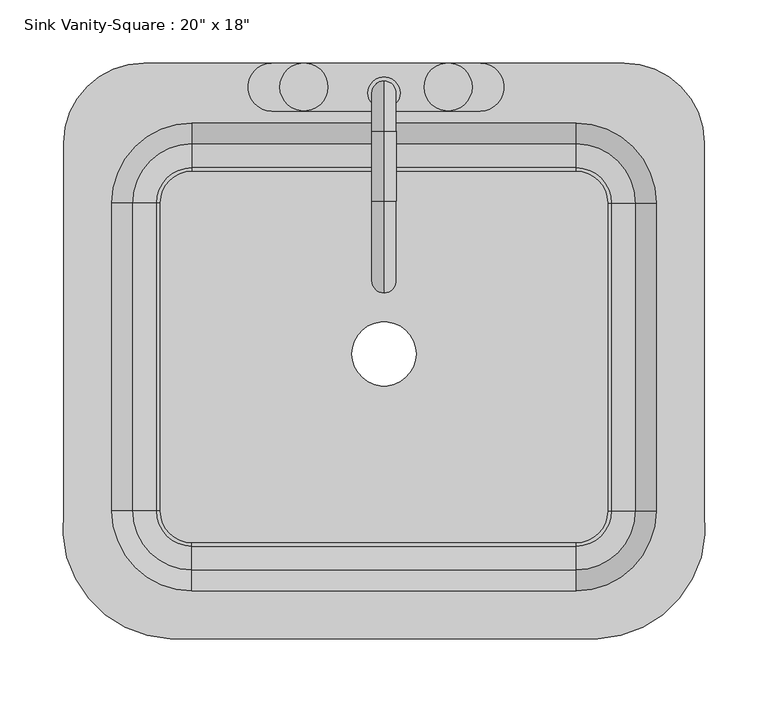
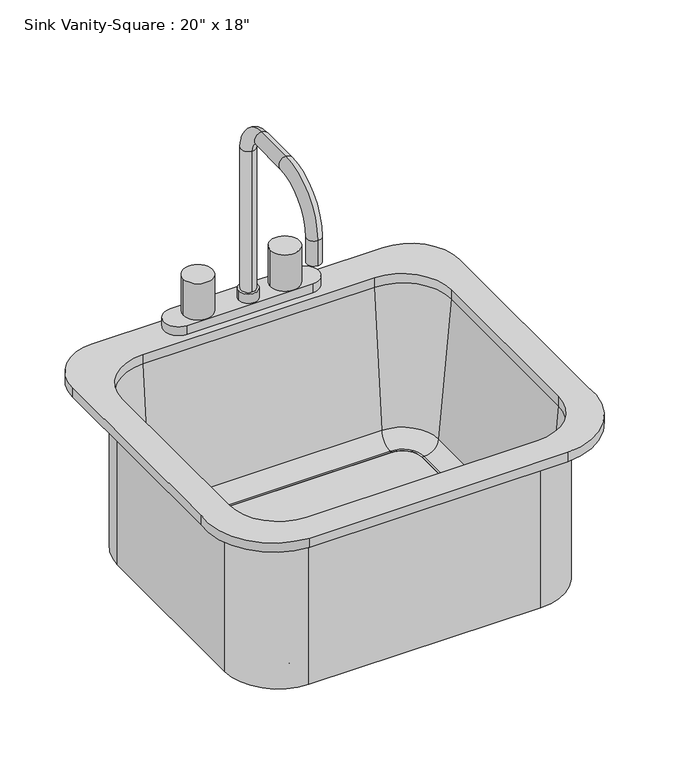
"""IFC4 building model written with IfcOpenShell, lengths in millimetres: flow terminal geometry."""

from ifc_helpers import new_model, si_unit, point, frame, frame_2d, origin, place, context, project, spatial, polyline, circle_curve, ellipse_curve, trimmed, segment, composite_curve, outline, extrude, source, transform, mapped, element, save
from ifc_brep_helpers import plane_surface, cylinder_surface, revolved_surface, advanced_brep


def flow_terminal_62a433f7(model_context):
    return source(origin(), model_context, "Body", "SolidModel", [
        advanced_brep(
        [(-153.9606923, -277.0545989, 800.1), (185.3391735, -277.0545989, 800.1), (269.6892406, -175.4545989, 800.1), (269.6892406, 116.6454011, 800.1), (206.1892406, 180.1454011, 800.1), (-174.8107593, 180.1454011, 800.1), (-238.3107593, 116.6454011, 800.1), (-238.3107593, -175.4545982, 800.1), (168.0892406, 132.5204011, 800.1), (231.5892406, 69.0204011, 800.1), (231.5892406, -175.4545989, 800.1), (168.0892406, -238.9545989, 800.1), (-136.7107594, -238.9545989, 800.1), (-200.2107594, -175.4545989, 800.1), (-200.2107594, 69.0204011, 800.1), (-136.7107594, 132.5204011, 800.1), (-153.9606923, -277.0545989, 787.4), (-238.3107593, -175.4545982, 787.4), (-238.3107593, 116.6454011, 787.4), (-174.8107593, 180.1454011, 787.4), (206.1892406, 180.1454011, 787.4), (269.6892406, 116.6454011, 787.4), (269.6892406, -175.4545989, 787.4), (185.3391735, -277.0545989, 787.4), (237.9392406, 69.0204011, 787.4), (168.0892406, 138.8704011, 787.4), (-136.7107594, 138.8704011, 787.4), (-206.5607594, 69.0204011, 787.4), (-206.5607594, -175.4545989, 787.4), (-136.7107594, -245.3045989, 787.4), (168.0892406, -245.3045989, 787.4), (237.9392406, -175.4545989, 787.4), (168.0892406, 132.5204011, 787.4), (231.5892406, 69.0204011, 787.4), (231.5892406, -175.4545989, 787.4), (168.0892406, -238.9545989, 787.4), (-136.7107594, -238.9545989, 787.4), (-200.2107594, -175.4545989, 787.4), (-200.2107594, 69.0204011, 787.4), (-136.7107594, 132.5204011, 787.4), (237.9392406, 69.0204011, 571.5), (168.0892406, 138.8704011, 571.5), (193.4892406, 69.0204011, 571.5), (168.0892406, 94.4204011, 571.5), (193.4892406, 69.0204011, 581.025), (168.0892406, 94.4204011, 581.025), (196.0776588, 69.0204011, 581.025), (168.0892406, 97.0088193, 581.025), (215.0551678, 69.0204011, 598.4146831), (168.0892406, 115.9863283, 598.4146831), (237.9392406, -175.4545989, 571.5), (193.4892406, -175.4545989, 571.5), (193.4892406, -175.4545989, 581.025), (196.0776588, -175.4545989, 581.025), (215.0551678, -175.4545989, 598.4146831), (168.0892406, -245.3045989, 571.5), (168.0892406, -200.8545989, 571.5), (168.0892406, -200.8545989, 581.025), (168.0892406, -203.4430171, 581.025), (168.0892406, -222.4205261, 598.4146831), (-136.7107594, -245.3045989, 571.5), (-136.7107594, -200.8545989, 571.5), (-136.7107594, -200.8545989, 581.025), (-136.7107594, -203.4430171, 581.025), (-136.7107594, -222.4205261, 598.4146831), (-206.5607594, -175.4545989, 571.5), (-162.1107594, -175.4545989, 571.5), (-162.1107594, -175.4545989, 581.025), (-164.6991776, -175.4545989, 581.025), (-183.6766866, -175.4545989, 598.4146831), (-206.5607594, 69.0204011, 571.5), (-162.1107594, 69.0204011, 571.5), (-162.1107594, 69.0204011, 581.025), (-164.6991776, 69.0204011, 581.025), (-183.6766866, 69.0204011, 598.4146831), (-136.7107594, 138.8704011, 571.5), (-136.7107594, 94.4204011, 571.5), (-136.7107594, 94.4204011, 581.025), (-136.7107594, 97.0088193, 581.025), (-136.7107594, 115.9863283, 598.4146831)],
        [
            (0, 1),
            (1, 2, circle_curve(frame((181.5319557, -188.0793432, 800.1), z_axis=(0.0, 0.0, 1.0), x_axis=(1.0, 0.0, 0.0)), 89.0566732)),
            (2, 3),
            (3, 4, circle_curve(frame((206.1892406, 116.6454011, 800.1), z_axis=(0.0, 0.0, 1.0), x_axis=(1.0, 0.0, 0.0)), 63.5)),
            (4, 5),
            (5, 6, circle_curve(frame((-174.8107593, 116.6454011, 800.1), z_axis=(0.0, 0.0, 1.0), x_axis=(1.0, 0.0, 0.0)), 63.5)),
            (6, 7),
            (7, 0, circle_curve(frame((-150.1534746, -188.0793432, 800.1), z_axis=(0.0, 0.0, 1.0), x_axis=(1.0, 0.0, 0.0)), 89.0566732)),
            (8, 9, circle_curve(frame((168.0892406, 69.0204011, 800.1), z_axis=(0.0, 0.0, -1.0), x_axis=(1.0, 0.0, 0.0)), 63.5)),
            (9, 10),
            (10, 11, circle_curve(frame((168.0892406, -175.4545989, 800.1), z_axis=(0.0, 0.0, -1.0), x_axis=(1.0, 0.0, 0.0)), 63.5)),
            (11, 12),
            (12, 13, circle_curve(frame((-136.7107594, -175.4545989, 800.1), z_axis=(0.0, 0.0, -1.0), x_axis=(1.0, 0.0, 0.0)), 63.5)),
            (13, 14),
            (14, 15, circle_curve(frame((-136.7107594, 69.0204011, 800.1), z_axis=(0.0, 0.0, -1.0), x_axis=(1.0, 0.0, 0.0)), 63.5)),
            (15, 8),
            (16, 17, circle_curve(frame((-150.1534746, -188.0793432, 787.4), z_axis=(0.0, 0.0, -1.0), x_axis=(1.0, 0.0, 0.0)), 89.0566732)),
            (17, 18),
            (18, 19, circle_curve(frame((-174.8107593, 116.6454011, 787.4), z_axis=(0.0, 0.0, -1.0), x_axis=(1.0, 0.0, 0.0)), 63.5)),
            (19, 20),
            (20, 21, circle_curve(frame((206.1892406, 116.6454011, 787.4), z_axis=(0.0, 0.0, -1.0), x_axis=(1.0, 0.0, 0.0)), 63.5)),
            (21, 22),
            (22, 23, circle_curve(frame((181.5319557, -188.0793432, 787.4), z_axis=(0.0, 0.0, -1.0), x_axis=(1.0, 0.0, 0.0)), 89.0566732)),
            (23, 16),
            (24, 25, circle_curve(frame((168.0892406, 69.0204011, 787.4), z_axis=(0.0, 0.0, 1.0), x_axis=(0.0, 1.0, 0.0)), 69.85)),
            (25, 26),
            (26, 27, circle_curve(frame((-136.7107594, 69.0204011, 787.4), z_axis=(0.0, 0.0, 1.0), x_axis=(-1.0, 0.0, 0.0)), 69.85)),
            (27, 28),
            (28, 29, circle_curve(frame((-136.7107594, -175.4545989, 787.4), z_axis=(0.0, 0.0, 1.0), x_axis=(0.0, -1.0, 0.0)), 69.85)),
            (29, 30),
            (30, 31, circle_curve(frame((168.0892406, -175.4545989, 787.4), z_axis=(0.0, 0.0, 1.0), x_axis=(1.0, 0.0, 0.0)), 69.85)),
            (31, 24),
            (0, 16),
            (23, 1),
            (22, 2),
            (21, 3),
            (20, 4),
            (19, 5),
            (18, 6),
            (17, 7),
            (8, 32),
            (32, 33, circle_curve(frame((168.0892406, 69.0204011, 787.4), z_axis=(0.0, 0.0, -1.0), x_axis=(1.0, 0.0, 0.0)), 63.5)),
            (33, 9),
            (33, 34),
            (34, 10),
            (34, 35, circle_curve(frame((168.0892406, -175.4545989, 787.4), z_axis=(0.0, 0.0, -1.0), x_axis=(1.0, 0.0, 0.0)), 63.5)),
            (35, 11),
            (35, 36),
            (36, 12),
            (36, 37, circle_curve(frame((-136.7107594, -175.4545989, 787.4), z_axis=(0.0, 0.0, -1.0), x_axis=(1.0, 0.0, 0.0)), 63.5)),
            (37, 13),
            (37, 38),
            (38, 14),
            (38, 39, circle_curve(frame((-136.7107594, 69.0204011, 787.4), z_axis=(0.0, 0.0, -1.0), x_axis=(1.0, 0.0, 0.0)), 63.5)),
            (39, 15),
            (39, 32),
            (40, 41, circle_curve(frame((168.0892406, 69.0204011, 571.5), z_axis=(0.0, 0.0, 1.0), x_axis=(0.0, 1.0, 0.0)), 69.85)),
            (41, 25),
            (24, 40),
            (40, 42),
            (42, 43, circle_curve(frame((168.0892406, 69.0204011, 571.5), z_axis=(0.0, 0.0, 1.0), x_axis=(0.0, 1.0, 0.0)), 25.4)),
            (43, 41),
            (42, 44),
            (44, 45, circle_curve(frame((168.0892406, 69.0204011, 581.025), z_axis=(0.0, 0.0, 1.0), x_axis=(0.0, 1.0, 0.0)), 25.4)),
            (45, 43),
            (44, 46),
            (46, 47, circle_curve(frame((168.0892406, 69.0204011, 581.025), z_axis=(0.0, 0.0, 1.0), x_axis=(0.0, 1.0, 0.0)), 27.9884182)),
            (47, 45),
            (46, 48, circle_curve(frame((196.0776588, 69.0204011, 600.075), z_axis=(0.0, -1.0, 0.0), x_axis=(1.0, 0.0, 0.0)), 19.05)),
            (48, 49, circle_curve(frame((168.0892406, 69.0204011, 598.4146831), z_axis=(0.0, 0.0, 1.0), x_axis=(0.0, 1.0, 0.0)), 46.9659272)),
            (49, 47, circle_curve(frame((168.0892406, 97.0088193, 600.075), z_axis=(-1.0, 0.0, 0.0), x_axis=(0.0, 1.0, 0.0)), 19.05)),
            (48, 33),
            (32, 49),
            (31, 50),
            (50, 40),
            (50, 51),
            (51, 42),
            (51, 52),
            (52, 44),
            (52, 53),
            (53, 46),
            (53, 54, circle_curve(frame((196.0776588, -175.4545989, 600.075), z_axis=(0.0, -1.0, 0.0), x_axis=(1.0, 0.0, 0.0)), 19.05)),
            (54, 48),
            (54, 34),
            (30, 55),
            (55, 50, circle_curve(frame((168.0892406, -175.4545989, 571.5), z_axis=(0.0, 0.0, 1.0), x_axis=(1.0, 0.0, 0.0)), 69.85)),
            (55, 56),
            (56, 51, circle_curve(frame((168.0892406, -175.4545989, 571.5), z_axis=(0.0, 0.0, 1.0), x_axis=(1.0, 0.0, 0.0)), 25.4)),
            (56, 57),
            (57, 52, circle_curve(frame((168.0892406, -175.4545989, 581.025), z_axis=(0.0, 0.0, 1.0), x_axis=(1.0, 0.0, 0.0)), 25.4)),
            (57, 58),
            (58, 53, circle_curve(frame((168.0892406, -175.4545989, 581.025), z_axis=(0.0, 0.0, 1.0), x_axis=(1.0, 0.0, 0.0)), 27.9884182)),
            (58, 59, circle_curve(frame((168.0892406, -203.4430171, 600.075), z_axis=(-1.0, 0.0, 0.0), x_axis=(0.0, -1.0, 0.0)), 19.05)),
            (59, 54, circle_curve(frame((168.0892406, -175.4545989, 598.4146831), z_axis=(0.0, 0.0, 1.0), x_axis=(1.0, 0.0, 0.0)), 46.9659272)),
            (59, 35),
            (29, 60),
            (60, 55),
            (60, 61),
            (61, 56),
            (61, 62),
            (62, 57),
            (62, 63),
            (63, 58),
            (63, 64, circle_curve(frame((-136.7107594, -203.4430171, 600.075), z_axis=(-1.0, 0.0, 0.0), x_axis=(0.0, -1.0, 0.0)), 19.05)),
            (64, 59),
            (64, 36),
            (28, 65),
            (65, 60, circle_curve(frame((-136.7107594, -175.4545989, 571.5), z_axis=(0.0, 0.0, 1.0), x_axis=(0.0, -1.0, 0.0)), 69.85)),
            (65, 66),
            (66, 61, circle_curve(frame((-136.7107594, -175.4545989, 571.5), z_axis=(0.0, 0.0, 1.0), x_axis=(0.0, -1.0, 0.0)), 25.4)),
            (66, 67),
            (67, 62, circle_curve(frame((-136.7107594, -175.4545989, 581.025), z_axis=(0.0, 0.0, 1.0), x_axis=(0.0, -1.0, 0.0)), 25.4)),
            (67, 68),
            (68, 63, circle_curve(frame((-136.7107594, -175.4545989, 581.025), z_axis=(0.0, 0.0, 1.0), x_axis=(0.0, -1.0, 0.0)), 27.9884182)),
            (68, 69, circle_curve(frame((-164.6991776, -175.4545989, 600.075), z_axis=(0.0, 1.0, 0.0), x_axis=(-1.0, 0.0, 0.0)), 19.05)),
            (69, 64, circle_curve(frame((-136.7107594, -175.4545989, 598.4146831), z_axis=(0.0, 0.0, 1.0), x_axis=(0.0, -1.0, 0.0)), 46.9659272)),
            (69, 37),
            (27, 70),
            (70, 65),
            (70, 71),
            (71, 66),
            (71, 72),
            (72, 67),
            (72, 73),
            (73, 68),
            (73, 74, circle_curve(frame((-164.6991776, 69.0204011, 600.075), z_axis=(0.0, 1.0, 0.0), x_axis=(-1.0, 0.0, 0.0)), 19.05)),
            (74, 69),
            (74, 38),
            (26, 75),
            (75, 70, circle_curve(frame((-136.7107594, 69.0204011, 571.5), z_axis=(0.0, 0.0, 1.0), x_axis=(-1.0, 0.0, 0.0)), 69.85)),
            (75, 76),
            (76, 71, circle_curve(frame((-136.7107594, 69.0204011, 571.5), z_axis=(0.0, 0.0, 1.0), x_axis=(-1.0, 0.0, 0.0)), 25.4)),
            (76, 77),
            (77, 72, circle_curve(frame((-136.7107594, 69.0204011, 581.025), z_axis=(0.0, 0.0, 1.0), x_axis=(-1.0, 0.0, 0.0)), 25.4)),
            (77, 78),
            (78, 73, circle_curve(frame((-136.7107594, 69.0204011, 581.025), z_axis=(0.0, 0.0, 1.0), x_axis=(-1.0, 0.0, 0.0)), 27.9884182)),
            (78, 79, circle_curve(frame((-136.7107594, 97.0088193, 600.075), z_axis=(1.0, 0.0, 0.0), x_axis=(0.0, 1.0, 0.0)), 19.05)),
            (79, 74, circle_curve(frame((-136.7107594, 69.0204011, 598.4146831), z_axis=(0.0, 0.0, 1.0), x_axis=(-1.0, 0.0, 0.0)), 46.9659272)),
            (79, 39),
            (41, 75),
            (43, 76),
            (45, 77),
            (47, 78),
            (49, 79),
        ],
        [
            plane_surface(frame((185.3391735, -277.0545989, 800.1), z_axis=(0.0, 0.0, 1.0), x_axis=(1.0, 0.0, 0.0))),
            plane_surface(frame((185.3391735, -277.0545989, 787.4), z_axis=(0.0, 0.0, -1.0), x_axis=(-1.0, 0.0, 0.0))),
            plane_surface(frame((-153.9606923, -277.0545989, 800.1), z_axis=(0.0, -1.0, 0.0), x_axis=(0.0, 0.0, -1.0))),
            cylinder_surface(frame((181.5319557, -188.0793432, 787.4), z_axis=(0.0, 0.0, 1.0), x_axis=(1.0, 0.0, 0.0)), 89.0566732),
            plane_surface(frame((269.6892406, -175.4545989, 800.1), z_axis=(1.0, 0.0, 0.0), x_axis=(0.0, 0.0, -1.0))),
            cylinder_surface(frame((206.1892406, 116.6454011, 787.4), z_axis=(0.0, 0.0, 1.0), x_axis=(1.0, 0.0, 0.0)), 63.5),
            plane_surface(frame((206.1892406, 180.1454011, 800.1), z_axis=(0.0, 1.0, 0.0), x_axis=(0.0, 0.0, -1.0))),
            cylinder_surface(frame((-174.8107593, 116.6454011, 787.4), z_axis=(0.0, 0.0, 1.0), x_axis=(1.0, 0.0, 0.0)), 63.5),
            plane_surface(frame((-238.3107593, 116.6454011, 800.1), z_axis=(-1.0, 0.0, 0.0), x_axis=(0.0, 0.0, -1.0))),
            cylinder_surface(frame((-150.1534746, -188.0793432, 787.4), z_axis=(0.0, 0.0, 1.0), x_axis=(1.0, 0.0, 0.0)), 89.0566732),
            revolved_surface(polyline([(231.5892406, 69.0204011, 787.4), (231.5892406, 69.0204011, 800.1)]), (168.0892406, 69.0204011, 0.0), (0.0, 0.0, -1.0)),
            plane_surface(frame((231.5892406, 69.0204011, 800.1), z_axis=(-1.0, 0.0, 0.0), x_axis=(0.0, 0.0, -1.0))),
            revolved_surface(polyline([(231.5892406, -175.4545989, 787.4), (231.5892406, -175.4545989, 800.1)]), (168.0892406, -175.4545989, 0.0), (0.0, 0.0, -1.0)),
            plane_surface(frame((168.0892406, -238.9545989, 800.1), z_axis=(0.0, 1.0, 0.0), x_axis=(0.0, 0.0, -1.0))),
            revolved_surface(polyline([(-73.2107594, -175.4545989, 787.4), (-73.2107594, -175.4545989, 800.1)]), (-136.7107594, -175.4545989, 0.0), (0.0, 0.0, -1.0)),
            plane_surface(frame((-200.2107594, -175.4545989, 800.1), z_axis=(1.0, 0.0, 0.0), x_axis=(0.0, 0.0, -1.0))),
            revolved_surface(polyline([(-73.2107594, 69.0204011, 787.4), (-73.2107594, 69.0204011, 800.1)]), (-136.7107594, 69.0204011, 0.0), (0.0, 0.0, -1.0)),
            plane_surface(frame((-136.7107594, 132.5204011, 800.1), z_axis=(0.0, -1.0, 0.0), x_axis=(0.0, 0.0, -1.0))),
            cylinder_surface(frame((168.0892406, 69.0204011, 0.0), z_axis=(0.0, 0.0, -1.0), x_axis=(0.0, 1.0, 0.0)), 69.85),
            plane_surface(frame((168.0892406, 69.0204011, 571.5), z_axis=(0.0, 0.0, -1.0), x_axis=(0.0, 1.0, 0.0))),
            revolved_surface(polyline([(168.0892406, 94.42040109999999, 571.5), (168.0892406, 94.42040109999999, 581.025)]), (168.0892406, 69.0204011, 0.0), (0.0, 0.0, -1.0)),
            plane_surface(frame((168.0892406, 69.0204011, 581.025), z_axis=(0.0, 0.0, 1.0), x_axis=(0.0, 1.0, 0.0))),
            revolved_surface(trimmed(ellipse_curve(frame((168.0892406, 97.0088193, 600.075), z_axis=(1.0, 0.0, 0.0), x_axis=(0.0, 1.0, 0.0)), 19.05, 19.05), [point((168.0892406, 97.0088193, 581.025))], [point((168.0892406, 115.9863283, 598.4146831))], True, "CARTESIAN"), (168.0892406, 69.0204011, 0.0), (0.0, 0.0, -1.0)),
            revolved_surface(polyline([(168.0892406, 115.9863283, 598.4146831), (168.0892406, 132.5204011, 787.4)]), (168.0892406, 69.0204011, 0.0), (0.0, 0.0, -1.0)),
            plane_surface(frame((237.9392406, 69.0204011, 787.4), z_axis=(1.0, 0.0, 0.0), x_axis=(0.0, -1.0, 0.0))),
            plane_surface(frame((237.9392406, 69.0204011, 571.5), z_axis=(0.0, 0.0, -1.0), x_axis=(0.0, -1.0, 0.0))),
            plane_surface(frame((193.4892406, 69.0204011, 571.5), z_axis=(-1.0, 0.0, 0.0), x_axis=(0.0, -1.0, 0.0))),
            plane_surface(frame((193.4892406, 69.0204011, 581.025), z_axis=(0.0, 0.0, 1.0), x_axis=(0.0, -1.0, 0.0))),
            revolved_surface(polyline([(215.1276588, -175.4545989, 600.075), (215.1276588, 69.0204011, 600.075)]), (196.0776588, 69.0204011, 600.075), (0.0, -1.0, 0.0)),
            plane_surface(frame((215.0551678, 69.0204011, 598.4146831), z_axis=(-0.9961946980917442, 0.0, 0.08715574274767397), x_axis=(0.0, -1.0, 0.0))),
            cylinder_surface(frame((168.0892406, -175.4545989, 0.0), z_axis=(0.0, 0.0, -1.0), x_axis=(1.0, 0.0, 0.0)), 69.85),
            plane_surface(frame((168.0892406, -175.4545989, 571.5), z_axis=(0.0, 0.0, -1.0), x_axis=(1.0, 0.0, 0.0))),
            revolved_surface(polyline([(193.48924060000002, -175.4545989, 571.5), (193.48924060000002, -175.4545989, 581.025)]), (168.0892406, -175.4545989, 0.0), (0.0, 0.0, -1.0)),
            plane_surface(frame((168.0892406, -175.4545989, 581.025), z_axis=(0.0, 0.0, 1.0), x_axis=(1.0, 0.0, 0.0))),
            revolved_surface(trimmed(ellipse_curve(frame((196.0776588, -175.4545989, 600.075), z_axis=(0.0, -1.0, 0.0), x_axis=(1.0, 0.0, 0.0)), 19.05, 19.05), [point((196.0776588, -175.4545989, 581.025))], [point((215.0551678, -175.4545989, 598.4146831))], True, "CARTESIAN"), (168.0892406, -175.4545989, 0.0), (0.0, 0.0, -1.0)),
            revolved_surface(polyline([(215.0551678, -175.4545989, 598.4146831), (231.5892406, -175.4545989, 787.4)]), (168.0892406, -175.4545989, 0.0), (0.0, 0.0, -1.0)),
            plane_surface(frame((168.0892406, -245.3045989, 787.4), z_axis=(0.0, -1.0, 0.0), x_axis=(-1.0, 0.0, 0.0))),
            plane_surface(frame((168.0892406, -245.3045989, 571.5), z_axis=(0.0, 0.0, -1.0), x_axis=(-1.0, 0.0, 0.0))),
            plane_surface(frame((168.0892406, -200.8545989, 571.5), z_axis=(0.0, 1.0, 0.0), x_axis=(-1.0, 0.0, 0.0))),
            plane_surface(frame((168.0892406, -200.8545989, 581.025), z_axis=(0.0, 0.0, 1.0), x_axis=(-1.0, 0.0, 0.0))),
            revolved_surface(polyline([(-136.7107594, -222.4930171, 600.075), (168.0892406, -222.4930171, 600.075)]), (168.0892406, -203.4430171, 600.075), (-1.0, 0.0, 0.0)),
            plane_surface(frame((168.0892406, -222.4205261, 598.4146831), z_axis=(0.0, 0.9961946980917442, 0.08715574274767397), x_axis=(-1.0, 0.0, 0.0))),
            cylinder_surface(frame((-136.7107594, -175.4545989, 0.0), z_axis=(0.0, 0.0, -1.0), x_axis=(0.0, -1.0, 0.0)), 69.85),
            plane_surface(frame((-136.7107594, -175.4545989, 571.5), z_axis=(0.0, 0.0, -1.0), x_axis=(0.0, -1.0, 0.0))),
            revolved_surface(polyline([(-136.7107594, -200.8545989, 571.5), (-136.7107594, -200.8545989, 581.025)]), (-136.7107594, -175.4545989, 0.0), (0.0, 0.0, -1.0)),
            plane_surface(frame((-136.7107594, -175.4545989, 581.025), z_axis=(0.0, 0.0, 1.0), x_axis=(0.0, -1.0, 0.0))),
            revolved_surface(trimmed(ellipse_curve(frame((-136.7107594, -203.4430171, 600.075), z_axis=(-1.0, 0.0, 0.0), x_axis=(0.0, -1.0, 0.0)), 19.05, 19.05), [point((-136.7107594, -203.4430171, 581.025))], [point((-136.7107594, -222.4205261, 598.4146831))], True, "CARTESIAN"), (-136.7107594, -175.4545989, 0.0), (0.0, 0.0, -1.0)),
            revolved_surface(polyline([(-136.7107594, -222.4205261, 598.4146831), (-136.7107594, -238.9545989, 787.4)]), (-136.7107594, -175.4545989, 0.0), (0.0, 0.0, -1.0)),
            plane_surface(frame((-206.5607594, -175.4545989, 787.4), z_axis=(-1.0, 0.0, 0.0), x_axis=(0.0, 1.0, 0.0))),
            plane_surface(frame((-206.5607594, -175.4545989, 571.5), z_axis=(0.0, 0.0, -1.0), x_axis=(0.0, 1.0, 0.0))),
            plane_surface(frame((-162.1107594, -175.4545989, 571.5), z_axis=(1.0, 0.0, 0.0), x_axis=(0.0, 1.0, 0.0))),
            plane_surface(frame((-162.1107594, -175.4545989, 581.025), z_axis=(0.0, 0.0, 1.0), x_axis=(0.0, 1.0, 0.0))),
            revolved_surface(polyline([(-183.74917760000002, 69.02040110000002, 600.075), (-183.74917760000002, -175.4545989, 600.075)]), (-164.6991776, -175.4545989, 600.075), (0.0, 1.0, 0.0)),
            plane_surface(frame((-183.6766866, -175.4545989, 598.4146831), z_axis=(0.9961946980917442, 0.0, 0.08715574274767397), x_axis=(0.0, 1.0, 0.0))),
            cylinder_surface(frame((-136.7107594, 69.0204011, 0.0), z_axis=(0.0, 0.0, -1.0), x_axis=(-1.0, 0.0, 0.0)), 69.85),
            plane_surface(frame((-136.7107594, 69.0204011, 571.5), z_axis=(0.0, 0.0, -1.0), x_axis=(-1.0, 0.0, 0.0))),
            revolved_surface(polyline([(-162.1107594, 69.0204011, 571.5), (-162.1107594, 69.0204011, 581.025)]), (-136.7107594, 69.0204011, 0.0), (0.0, 0.0, -1.0)),
            plane_surface(frame((-136.7107594, 69.0204011, 581.025), z_axis=(0.0, 0.0, 1.0), x_axis=(-1.0, 0.0, 0.0))),
            revolved_surface(trimmed(ellipse_curve(frame((-164.6991776, 69.0204011, 600.075), z_axis=(0.0, 1.0, 0.0), x_axis=(-1.0, 0.0, 0.0)), 19.05, 19.05), [point((-164.6991776, 69.0204011, 581.025))], [point((-183.6766866, 69.0204011, 598.4146831))], True, "CARTESIAN"), (-136.7107594, 69.0204011, 0.0), (0.0, 0.0, -1.0)),
            revolved_surface(polyline([(-183.6766866, 69.0204011, 598.4146831), (-200.2107594, 69.0204011, 787.4)]), (-136.7107594, 69.0204011, 0.0), (0.0, 0.0, -1.0)),
            plane_surface(frame((-136.7107594, 138.8704011, 787.4), z_axis=(0.0, 1.0, 0.0), x_axis=(1.0, 0.0, 0.0))),
            plane_surface(frame((-136.7107594, 138.8704011, 571.5), z_axis=(0.0, 0.0, -1.0), x_axis=(1.0, 0.0, 0.0))),
            plane_surface(frame((-136.7107594, 94.4204011, 571.5), z_axis=(0.0, -1.0, 0.0), x_axis=(1.0, 0.0, 0.0))),
            plane_surface(frame((-136.7107594, 94.4204011, 581.025), z_axis=(0.0, 0.0, 1.0), x_axis=(1.0, 0.0, 0.0))),
            revolved_surface(polyline([(168.0892406, 116.0588193, 600.075), (-136.7107594, 116.0588193, 600.075)]), (-136.7107594, 97.0088193, 600.075), (1.0, 0.0, 0.0)),
            plane_surface(frame((-136.7107594, 115.9863283, 598.4146831), z_axis=(0.0, -0.9961946980917442, 0.08715574274767397), x_axis=(1.0, 0.0, 0.0))),
        ],
        [
            (0, [[1, 2, 3, 4, 5, 6, 7, 8], [9, 10, 11, 12, 13, 14, 15, 16]]),
            (1, [[17, 18, 19, 20, 21, 22, 23, 24], [25, 26, 27, 28, 29, 30, 31, 32]]),
            (2, [[-1, 33, -24, 34]]),
            (3, [[-2, -34, -23, 35]]),
            (4, [[-3, -35, -22, 36]]),
            (5, [[-4, -36, -21, 37]]),
            (6, [[-5, -37, -20, 38]]),
            (7, [[-6, -38, -19, 39]]),
            (8, [[-7, -39, -18, 40]]),
            (9, [[-8, -40, -17, -33]]),
            (10, [[-9, 41, 42, 43]]),
            (11, [[-10, -43, 44, 45]]),
            (12, [[-11, -45, 46, 47]]),
            (13, [[-12, -47, 48, 49]]),
            (14, [[-13, -49, 50, 51]]),
            (15, [[-14, -51, 52, 53]]),
            (16, [[-15, -53, 54, 55]]),
            (17, [[-16, -55, 56, -41]]),
            (18, [[57, 58, -25, 59]]),
            (19, [[-57, 60, 61, 62]]),
            (20, [[-61, 63, 64, 65]]),
            (21, [[-64, 66, 67, 68]]),
            (22, [[-67, 69, 70, 71]]),
            (23, [[-70, 72, -42, 73]]),
            (24, [[-59, -32, 74, 75]]),
            (25, [[-60, -75, 76, 77]]),
            (26, [[-63, -77, 78, 79]]),
            (27, [[-66, -79, 80, 81]]),
            (28, [[-69, -81, 82, 83]]),
            (29, [[-72, -83, 84, -44]]),
            (30, [[-74, -31, 85, 86]]),
            (31, [[-76, -86, 87, 88]]),
            (32, [[-78, -88, 89, 90]]),
            (33, [[-80, -90, 91, 92]]),
            (34, [[-82, -92, 93, 94]]),
            (35, [[-84, -94, 95, -46]]),
            (36, [[-85, -30, 96, 97]]),
            (37, [[-87, -97, 98, 99]]),
            (38, [[-89, -99, 100, 101]]),
            (39, [[-91, -101, 102, 103]]),
            (40, [[-93, -103, 104, 105]]),
            (41, [[-95, -105, 106, -48]]),
            (42, [[-96, -29, 107, 108]]),
            (43, [[-98, -108, 109, 110]]),
            (44, [[-100, -110, 111, 112]]),
            (45, [[-102, -112, 113, 114]]),
            (46, [[-104, -114, 115, 116]]),
            (47, [[-106, -116, 117, -50]]),
            (48, [[-107, -28, 118, 119]]),
            (49, [[-109, -119, 120, 121]]),
            (50, [[-111, -121, 122, 123]]),
            (51, [[-113, -123, 124, 125]]),
            (52, [[-115, -125, 126, 127]]),
            (53, [[-117, -127, 128, -52]]),
            (54, [[-118, -27, 129, 130]]),
            (55, [[-120, -130, 131, 132]]),
            (56, [[-122, -132, 133, 134]]),
            (57, [[-124, -134, 135, 136]]),
            (58, [[-126, -136, 137, 138]]),
            (59, [[-128, -138, 139, -54]]),
            (60, [[-58, 140, -129, -26]]),
            (61, [[-62, 141, -131, -140]]),
            (62, [[-65, 142, -133, -141]]),
            (63, [[-68, 143, -135, -142]]),
            (64, [[-71, 144, -137, -143]]),
            (65, [[-73, -56, -139, -144]]),
        ],
    ),
        advanced_brep(
        [(91.8892406, 180.1454011, 800.1), (91.8892406, 142.0454011, 800.1), (-73.2107594, 142.0454011, 800.1), (-73.2107594, 180.1454011, 800.1), (15.6892406, 165.8579011, 1020.7625), (15.6892406, 146.8079011, 1020.7625), (15.6892406, 146.8079011, 825.5), (15.6892406, 165.8579011, 825.5), (15.6892406, 126.1704011, 1060.45), (15.6892406, 126.1704011, 1041.4), (15.6892406, 70.6079011, 1060.45), (15.6892406, 70.6079011, 1041.4), (15.6892406, -2.4170989, 987.425), (15.6892406, 16.6329011, 987.425), (15.6892406, -2.4170989, 952.5), (15.6892406, 16.6329011, 952.5), (2.9892406, 156.3329011, 825.5), (28.3892406, 156.3329011, 825.5), (2.9892406, 156.3329011, 812.8), (28.3892406, 156.3329011, 812.8), (91.8892406, 180.1454011, 812.8), (-73.2107594, 180.1454011, 812.8), (-73.2107594, 142.0454011, 812.8), (91.8892406, 142.0454011, 812.8)],
        [
            (0, 1, circle_curve(frame((91.8892406, 161.0954011, 800.1), z_axis=(0.0, 0.0, -1.0), x_axis=(1.0, 0.0, 0.0)), 19.05)),
            (1, 2),
            (2, 3, circle_curve(frame((-73.2107594, 161.0954011, 800.1), z_axis=(0.0, 0.0, -1.0), x_axis=(1.0, 0.0, 0.0)), 19.05)),
            (3, 0),
            (4, 5, circle_curve(frame((15.6892406, 156.3329011, 1020.7625), z_axis=(0.0, 0.0, -1.0), x_axis=(0.0, -1.0, 0.0)), 9.525)),
            (5, 6),
            (6, 7, circle_curve(frame((15.6892406, 156.3329011, 825.5), z_axis=(0.0, 0.0, 1.0), x_axis=(0.0, -1.0, 0.0)), 9.525)),
            (7, 4),
            (5, 4, circle_curve(frame((15.6892406, 156.3329011, 1020.7625), z_axis=(0.0, 0.0, -1.0), x_axis=(0.0, -1.0, 0.0)), 9.525)),
            (7, 6, circle_curve(frame((15.6892406, 156.3329011, 825.5), z_axis=(0.0, 0.0, 1.0), x_axis=(0.0, -1.0, 0.0)), 9.525)),
            (4, 8, circle_curve(frame((15.6892406, 126.1704011, 1020.7625), z_axis=(1.0, 0.0, 0.0), x_axis=(0.0, 1.0, 0.0)), 39.6875)),
            (8, 9, circle_curve(frame((15.6892406, 126.1704011, 1050.925), z_axis=(0.0, 1.0, 0.0), x_axis=(0.0, 0.0, -1.0)), 9.525)),
            (9, 5, circle_curve(frame((15.6892406, 126.1704011, 1020.7625), z_axis=(-1.0, 0.0, 0.0), x_axis=(0.0, 1.0, 0.0)), 20.6375)),
            (9, 8, circle_curve(frame((15.6892406, 126.1704011, 1050.925), z_axis=(0.0, 1.0, 0.0), x_axis=(0.0, 0.0, -1.0)), 9.525)),
            (8, 10),
            (10, 11, circle_curve(frame((15.6892406, 70.6079011, 1050.925), z_axis=(0.0, 1.0, 0.0), x_axis=(0.0, 0.0, -1.0)), 9.525)),
            (11, 9),
            (11, 10, circle_curve(frame((15.6892406, 70.6079011, 1050.925), z_axis=(0.0, 1.0, 0.0), x_axis=(0.0, 0.0, -1.0)), 9.525)),
            (10, 12, circle_curve(frame((15.6892406, 70.6079011, 987.425), z_axis=(1.0, 0.0, 0.0), x_axis=(0.0, 0.0, 1.0)), 73.025)),
            (12, 13, circle_curve(frame((15.6892406, 7.1079011, 987.425), z_axis=(0.0, 0.0, 1.0), x_axis=(0.0, 1.0, 0.0)), 9.525)),
            (13, 11, circle_curve(frame((15.6892406, 70.6079011, 987.425), z_axis=(-1.0, 0.0, 0.0), x_axis=(0.0, 0.0, 1.0)), 53.975)),
            (13, 12, circle_curve(frame((15.6892406, 7.1079011, 987.425), z_axis=(0.0, 0.0, 1.0), x_axis=(0.0, 1.0, 0.0)), 9.525)),
            (14, 15, circle_curve(frame((15.6892406, 7.1079011, 952.5), z_axis=(0.0, 0.0, -1.0), x_axis=(0.0, 1.0, 0.0)), 9.525)),
            (15, 14, circle_curve(frame((15.6892406, 7.1079011, 952.5), z_axis=(0.0, 0.0, -1.0), x_axis=(0.0, 1.0, 0.0)), 9.525)),
            (12, 14),
            (15, 13),
            (16, 17, circle_curve(frame((15.6892406, 156.3329011, 825.5), z_axis=(0.0, 0.0, 1.0), x_axis=(1.0, 0.0, 0.0)), 12.7)),
            (17, 16, circle_curve(frame((15.6892406, 156.3329011, 825.5), z_axis=(0.0, 0.0, 1.0), x_axis=(1.0, 0.0, 0.0)), 12.7)),
            (16, 18),
            (18, 19, circle_curve(frame((15.6892406, 156.3329011, 812.8), z_axis=(0.0, 0.0, 1.0), x_axis=(1.0, 0.0, 0.0)), 12.7)),
            (19, 17),
            (19, 18, circle_curve(frame((15.6892406, 156.3329011, 812.8), z_axis=(0.0, 0.0, 1.0), x_axis=(1.0, 0.0, 0.0)), 12.7)),
            (20, 21),
            (21, 22, circle_curve(frame((-73.2107594, 161.0954011, 812.8), z_axis=(0.0, 0.0, 1.0), x_axis=(1.0, 0.0, 0.0)), 19.05)),
            (22, 23),
            (23, 20, circle_curve(frame((91.8892406, 161.0954011, 812.8), z_axis=(0.0, 0.0, 1.0), x_axis=(1.0, 0.0, 0.0)), 19.05)),
            (20, 0),
            (3, 21),
            (2, 22),
            (1, 23),
        ],
        [
            plane_surface(frame((15.6892406, 146.8079011, 800.1), z_axis=(0.0, 0.0, -1.0), x_axis=(1.0, 0.0, 0.0))),
            cylinder_surface(frame((15.6892406, 156.3329011, 800.1), z_axis=(0.0, 0.0, -1.0), x_axis=(0.0, -1.0, 0.0)), 9.525),
            revolved_surface(trimmed(ellipse_curve(frame((15.6892406, 156.3329011, 1020.7625), z_axis=(0.0, 0.0, -1.0), x_axis=(0.0, -1.0, 0.0)), 9.525, 9.525), [point((15.6892406, 165.8579011, 1020.7625))], [point((15.6892406, 146.8079011, 1020.7625))], True, "CARTESIAN"), (15.6892406, 126.1704011, 1020.7625), (1.0, 0.0, 0.0)),
            revolved_surface(trimmed(ellipse_curve(frame((15.6892406, 156.3329011, 1020.7625), z_axis=(0.0, 0.0, -1.0), x_axis=(0.0, -1.0, 0.0)), 9.525, 9.525), [point((15.6892406, 146.8079011, 1020.7625))], [point((15.6892406, 165.8579011, 1020.7625))], True, "CARTESIAN"), (15.6892406, 126.1704011, 1020.7625), (1.0, 0.0, 0.0)),
            cylinder_surface(frame((15.6892406, 126.1704011, 1050.925), z_axis=(0.0, 1.0, 0.0), x_axis=(0.0, 0.0, -1.0)), 9.525),
            revolved_surface(trimmed(ellipse_curve(frame((15.6892406, 70.6079011, 1050.925), z_axis=(0.0, 1.0, 0.0), x_axis=(0.0, 0.0, -1.0)), 9.525, 9.525), [point((15.6892406, 70.6079011, 1060.45))], [point((15.6892406, 70.6079011, 1041.4))], True, "CARTESIAN"), (15.6892406, 70.6079011, 987.425), (1.0, 0.0, 0.0)),
            revolved_surface(trimmed(ellipse_curve(frame((15.6892406, 70.6079011, 1050.925), z_axis=(0.0, 1.0, 0.0), x_axis=(0.0, 0.0, -1.0)), 9.525, 9.525), [point((15.6892406, 70.6079011, 1041.4))], [point((15.6892406, 70.6079011, 1060.45))], True, "CARTESIAN"), (15.6892406, 70.6079011, 987.425), (1.0, 0.0, 0.0)),
            plane_surface(frame((15.6892406, -2.4170989, 952.5), z_axis=(0.0, 0.0, -1.0), x_axis=(-1.0, 0.0, 0.0))),
            cylinder_surface(frame((15.6892406, 7.1079011, 987.425), z_axis=(0.0, 0.0, 1.0), x_axis=(0.0, 1.0, 0.0)), 9.525),
            plane_surface(frame((28.3892406, 156.3329011, 825.5), z_axis=(0.0, 0.0, 1.0), x_axis=(0.0, 1.0, 0.0))),
            cylinder_surface(frame((15.6892406, 156.3329011, 812.8), z_axis=(0.0, 0.0, 1.0), x_axis=(1.0, 0.0, 0.0)), 12.7),
            plane_surface(frame((-73.2107594, 180.1454011, 812.8), z_axis=(0.0, 0.0, 1.0), x_axis=(-1.0, 0.0, 0.0))),
            plane_surface(frame((91.8892406, 180.1454011, 812.8), z_axis=(0.0, 1.0, 0.0), x_axis=(0.0, 0.0, -1.0))),
            cylinder_surface(frame((-73.2107594, 161.0954011, 800.1), z_axis=(0.0, 0.0, 1.0), x_axis=(1.0, 0.0, 0.0)), 19.05),
            plane_surface(frame((-73.2107594, 142.0454011, 812.8), z_axis=(0.0, -1.0, 0.0), x_axis=(0.0, 0.0, -1.0))),
            cylinder_surface(frame((91.8892406, 161.0954011, 800.1), z_axis=(0.0, 0.0, 1.0), x_axis=(1.0, 0.0, 0.0)), 19.05),
        ],
        [
            (0, [[1, 2, 3, 4]]),
            (1, [[5, 6, 7, 8]]),
            (1, [[9, -8, 10, -6]]),
            (2, [[-5, 11, 12, 13]]),
            (3, [[-9, -13, 14, -11]]),
            (4, [[-12, 15, 16, 17]]),
            (4, [[-14, -17, 18, -15]]),
            (5, [[-16, 19, 20, 21]]),
            (6, [[-18, -21, 22, -19]]),
            (7, [[23, 24]]),
            (8, [[-20, 25, -24, 26]]),
            (8, [[-22, -26, -23, -25]]),
            (9, [[27, 28], [-7, -10]]),
            (10, [[-27, 29, 30, 31]]),
            (10, [[-28, -31, 32, -29]]),
            (11, [[33, 34, 35, 36], [-30, -32]]),
            (12, [[-33, 37, -4, 38]]),
            (13, [[-34, -38, -3, 39]]),
            (14, [[-35, -39, -2, 40]]),
            (15, [[-36, -40, -1, -37]]),
        ],
    ),
        extrude(outline(composite_curve([segment(trimmed(circle_curve(frame_2d((-47.8107594, 161.0954011)), 19.05), [point((-66.8607594, 161.0954011))], [point((-28.7607594, 161.0954011))], False, "CARTESIAN"), True, "CONTINUOUS"), segment(trimmed(circle_curve(frame_2d((-47.8107594, 161.0954011)), 19.05), [point((-28.7607594, 161.0954011))], [point((-66.8607594, 161.0954011))], False, "CARTESIAN"), True, "CONTINUOUS")], self_intersect=False)), frame((0.0, 0.0, 812.8), z_axis=(0.0, 0.0, 1.0), x_axis=(1.0, 0.0, 0.0)), (0.0, 0.0, 1.0), 50.8),
        extrude(outline(composite_curve([segment(trimmed(circle_curve(frame_2d((66.4892406, 161.0954011)), 19.05), [point((47.4392406, 161.0954011))], [point((85.5392406, 161.0954011))], False, "CARTESIAN"), True, "CONTINUOUS"), segment(trimmed(circle_curve(frame_2d((66.4892406, 161.0954011)), 19.05), [point((85.5392406, 161.0954011))], [point((47.4392406, 161.0954011))], False, "CARTESIAN"), True, "CONTINUOUS")], self_intersect=False)), frame((0.0, 0.0, 812.8), z_axis=(0.0, 0.0, 1.0), x_axis=(1.0, 0.0, 0.0)), (0.0, 0.0, 1.0), 50.8),
        extrude(outline(composite_curve([segment(trimmed(circle_curve(frame_2d((168.0892406, 69.0204011)), 25.4), [point((168.0892406, 94.4204011))], [point((193.4892406, 69.0204011))], False, "CARTESIAN"), True, "CONTINUOUS"), segment(polyline([(193.4892406, 69.0204011), (193.4892406, -175.4545989)]), True, "CONTINUOUS"), segment(trimmed(circle_curve(frame_2d((168.0892406, -175.4545989)), 25.4), [point((193.4892406, -175.4545989))], [point((168.0892406, -200.8545989))], False, "CARTESIAN"), True, "CONTINUOUS"), segment(polyline([(168.0892406, -200.8545989), (-136.7107594, -200.8545989)]), True, "CONTINUOUS"), segment(trimmed(circle_curve(frame_2d((-136.7107594, -175.4545989)), 25.4), [point((-136.7107594, -200.8545989))], [point((-162.1107594, -175.4545989))], False, "CARTESIAN"), True, "CONTINUOUS"), segment(polyline([(-162.1107594, -175.4545989), (-162.1107594, 69.0204011)]), True, "CONTINUOUS"), segment(trimmed(circle_curve(frame_2d((-136.7107594, 69.0204011)), 25.4), [point((-162.1107594, 69.0204011))], [point((-136.7107594, 94.4204011))], False, "CARTESIAN"), True, "CONTINUOUS"), segment(polyline([(-136.7107594, 94.4204011), (168.0892406, 94.4204011)]), True, "CONTINUOUS")], self_intersect=False), holes=[composite_curve([segment(trimmed(circle_curve(frame_2d((15.6892406, -50.8)), 25.4), [point((-9.7107594, -50.8))], [point((41.0892406, -50.8))], True, "CARTESIAN"), True, "CONTINUOUS"), segment(trimmed(circle_curve(frame_2d((15.6892406, -50.8)), 25.4), [point((41.0892406, -50.8))], [point((-9.7107594, -50.8))], True, "CARTESIAN"), True, "CONTINUOUS")], self_intersect=False)]), frame((0.0, 0.0, 571.5), z_axis=(0.0, 0.0, 1.0), x_axis=(1.0, 0.0, 0.0)), (0.0, 0.0, 1.0), 9.525),
    ])


if __name__ == "__main__":
    model = new_model("IFC4")
    model_context = context("Model", 3, world=origin())
    ifc_project = project(units=[si_unit("LENGTHUNIT", "METRE", prefix="MILLI")], contexts=[model_context])
    site = spatial("IfcSite", under=ifc_project)
    building = spatial("IfcBuilding", under=site)
    placement = place(None, origin())
    flow_terminal_shape = flow_terminal_62a433f7(model_context)
    element("IfcFlowTerminal", 1, ObjectType="Sink Vanity-Square : 20\" x 18\"", at=placement, inside=building, context=model_context, shape_type="MappedRepresentation", body=[
        mapped(flow_terminal_shape, transform((0.0, 0.0, 0.0), x_axis=(1.0, 0.0, 0.0), y_axis=(0.0, 1.0, 0.0), z_axis=(0.0, 0.0, 1.0))),
    ])
    save(model, "model.ifc")

# Revit data of these elements
# Type "Sink Vanity-Square : 20\" x 18\""
#   Assembly Code = "D2010400"
#   Counter Height = 2' - 7"
#   Depth = 1' - 6"
#   Width = 1' - 8"
#   Basin Material = Porcelain, Linen
#   Faucet Material = Steel, Polished
#   Default Elevation = 0
# Element 1 (IfcFlowTerminal, "Sink Vanity-Square : 20\" x 18\"")
#   Materials on its faces: "Porcelain, Linen", "Steel, Polished"
# Materials
#   "Porcelain, Linen": class "Ceramic", colour RGB 249 239 230, transparency 0, Description = "Porcelain, linen", Cost = 0
#   "Steel, Polished": class "Metal", colour RGB 192 192 192, transparency 0, Description = "Polished steel", Cost = 0
